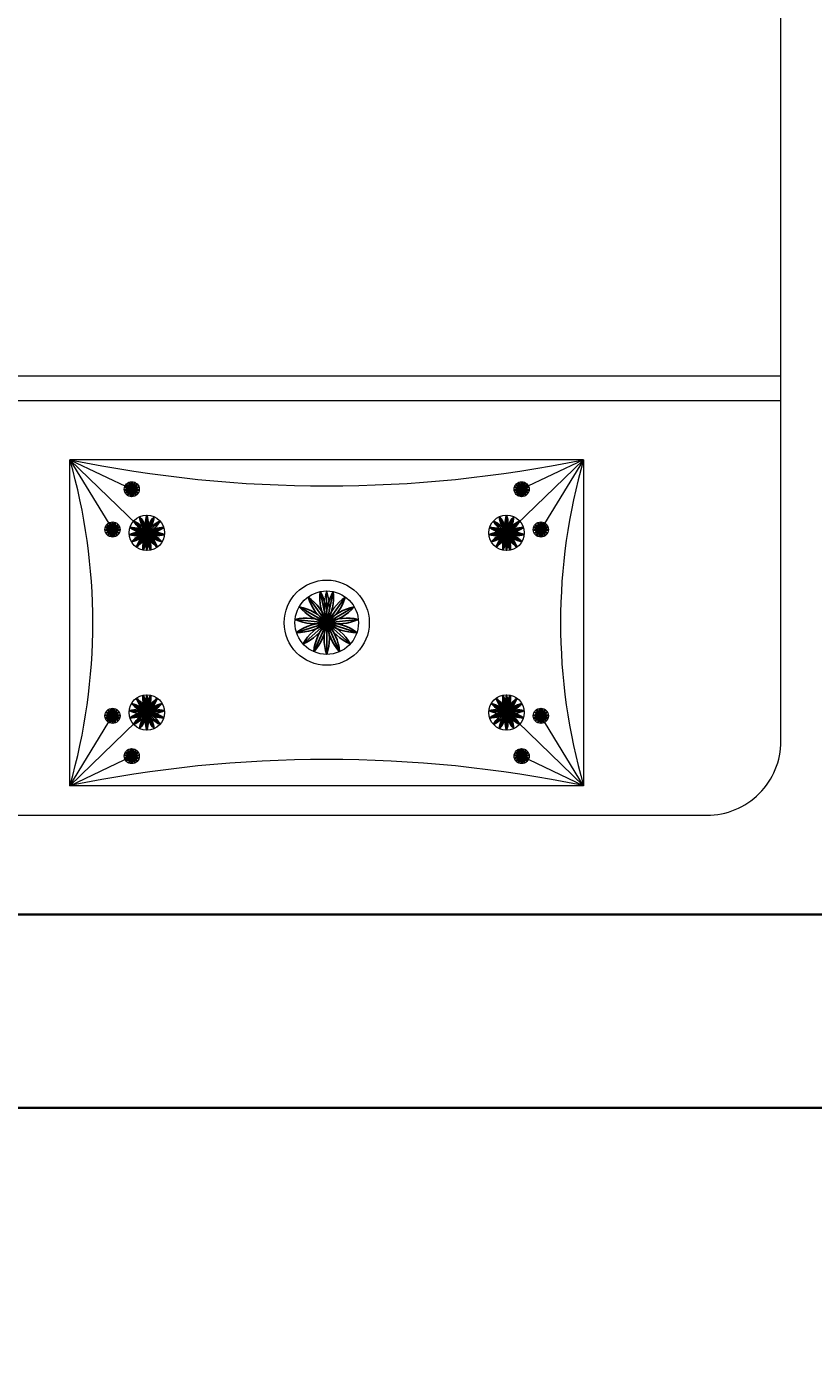
# Model space of a CAD drawing. Units: inches. Extents: x -61 to 1599, y -1316 to 257.
# Tile 187 of 204: x 1126 to 1163, y -454 to -391. Entities that reach past the tile are written whole.
import ezdxf

# ---------------------------------------------------------------- set-up
doc = ezdxf.new("R2010")
doc.units = ezdxf.units.IN
doc.header["$MEASUREMENT"] = 0
for name, color, linetype, lineweight in [('A-ANNO-DIMS', 2, 'Continuous', 18), ('FURNITURE', 83, 'Continuous', 18), ('WALLS', 4, 'Continuous', 35)]:
    doc.layers.add(name, color=color, linetype=linetype, lineweight=lineweight)
doc.layers.add('LT', color=8, linetype='Continuous')
doc.styles.get("Standard").update_dxf_attribs({"font": 'arial.ttf'})
doc.dimstyles.get("Standard").update_dxf_attribs({"dimtxt": 0.18, "dimasz": 0.18, "dimexe": 0.18, "dimexo": 0.0625, "dimgap": 0.09, "dimtad": 0, "dimtih": 1, "dimtoh": 1, "dimdec": 0, "dimzin": 0, "dimdsep": 46, "dimlunit": 3, "dimtxsty": 'Standard', "dimcen": 0.09, "dimadec": 0, "dimazin": 0, "dimtfac": 1, "dimtdec": 0, "dimtofl": 0, "dimtmove": 0, "dimatfit": 3, "dimfxl": 1, "dimtolj": 1, "dimtzin": 0, "dimarcsym": 0})

# ---------------------------------------------------------------- blocks, each defined once
blk = doc.blocks.new('*U3')
at = {"layer": 'LT'}
blk.add_line((0, 0.175), (0, -0.175), dxfattribs=at)
for centre, start, end in [((0.509, 0), 160.9983, 199.0017), ((-0.509, 0), 340.9983, 19.0017)]:
    blk.add_arc(centre, 0.539, start, end, dxfattribs=at)
blk = doc.blocks.new('*U4')
at = {"layer": 'LT', "transparency": 16777216}
for p, rotation in [((-66.649, -18.828), 96), ((-66.642, -18.755), 72), ((-66.627, -18.897), 120), ((-66.605, -18.692), 48.00000000000001), ((-66.578, -18.951), 144), ((-66.546, -18.649), 24), ((-66.512, -18.981), 168.0000000000001), ((-66.439, -18.981), 192), ((-66.404, -18.649), 336.0000000000001), ((-66.372, -18.951), 216), ((-66.345, -18.692), 312), ((-66.323, -18.897), 240), ((-66.308, -18.755), 288.0000000000001), ((-66.301, -18.828), 264)]:
    blk.add_blockref('*U3', p, dxfattribs=dict(at, rotation=rotation))
blk.add_blockref('*U3', (-66.475, -18.634), dxfattribs=at)
blk = doc.blocks.new('*U20')
at = {"layer": 'LT'}
blk.add_line((0, 0.175), (0, -0.175), dxfattribs=at)
for centre, start, end in [((0.509, 0), 160.9983, 199.0017), ((-0.509, 0), 340.9983, 19.0017)]:
    blk.add_arc(centre, 0.539, start, end, dxfattribs=at)
blk = doc.blocks.new('*U21')
at = {"layer": 'LT', "transparency": 16777216}
for p, rotation in [((-66.649, -18.828), 96), ((-66.642, -18.755), 72), ((-66.627, -18.897), 120), ((-66.605, -18.692), 48.00000000000001), ((-66.578, -18.951), 144), ((-66.546, -18.649), 24), ((-66.512, -18.981), 168.0000000000001), ((-66.439, -18.981), 192), ((-66.404, -18.649), 336.0000000000001), ((-66.372, -18.951), 216), ((-66.345, -18.692), 312), ((-66.323, -18.897), 240), ((-66.308, -18.755), 288.0000000000001), ((-66.301, -18.828), 264)]:
    blk.add_blockref('*U20', p, dxfattribs=dict(at, rotation=rotation))
blk.add_blockref('*U20', (-66.475, -18.634), dxfattribs=at)
blk = doc.blocks.new('*U52')
at = {"layer": 'LT'}
blk.add_line((0, 0.175), (0, -0.175), dxfattribs=at)
for centre, start, end in [((0.509, 0), 160.9983, 199.0017), ((-0.509, 0), 340.9983, 19.0017)]:
    blk.add_arc(centre, 0.539, start, end, dxfattribs=at)
blk = doc.blocks.new('*U53')
at = {"layer": 'LT', "transparency": 16777216}
for p, rotation in [((-66.649, -18.828), 96), ((-66.642, -18.755), 72), ((-66.627, -18.897), 120), ((-66.605, -18.692), 48.00000000000001), ((-66.578, -18.951), 144), ((-66.546, -18.649), 24), ((-66.512, -18.981), 168.0000000000001), ((-66.439, -18.981), 192), ((-66.404, -18.649), 336.0000000000001), ((-66.372, -18.951), 216), ((-66.345, -18.692), 312), ((-66.323, -18.897), 240), ((-66.308, -18.755), 288.0000000000001), ((-66.301, -18.828), 264)]:
    blk.add_blockref('*U52', p, dxfattribs=dict(at, rotation=rotation))
blk.add_blockref('*U52', (-66.475, -18.634), dxfattribs=at)
blk = doc.blocks.new('*U29')
at = {"layer": 'LT'}
blk.add_line((0, 0.175), (0, -0.175), dxfattribs=at)
for centre, start, end in [((0.509, 0), 160.9983, 199.0017), ((-0.509, 0), 340.9983, 19.0017)]:
    blk.add_arc(centre, 0.539, start, end, dxfattribs=at)
blk = doc.blocks.new('*U30')
at = {"layer": 'LT', "transparency": 16777216}
for p, rotation in [((-66.649, -18.828), 96), ((-66.642, -18.755), 72), ((-66.627, -18.897), 120), ((-66.605, -18.692), 48.00000000000001), ((-66.578, -18.951), 144), ((-66.546, -18.649), 24), ((-66.512, -18.981), 168.0000000000001), ((-66.439, -18.981), 192), ((-66.404, -18.649), 336.0000000000001), ((-66.372, -18.951), 216), ((-66.345, -18.692), 312), ((-66.323, -18.897), 240), ((-66.308, -18.755), 288.0000000000001), ((-66.301, -18.828), 264)]:
    blk.add_blockref('*U29', p, dxfattribs=dict(at, rotation=rotation))
blk.add_blockref('*U29', (-66.475, -18.634), dxfattribs=at)
blk = doc.blocks.new('*U5')
at = {"layer": 'LT'}
blk.add_line((0, 0.412), (0, -0.412), dxfattribs=at)
for centre, start, end in [((1.198, 0), 160.9983, 199.0017), ((-1.198, 0), 340.9983, 19.0017)]:
    blk.add_arc(centre, 1.267, start, end, dxfattribs=at)
blk = doc.blocks.new('*U47')
at = {"layer": 'LT', "transparency": 16777216}
for p, rotation in [((-156.639, -43.959), 48.00000000000001), ((-156.501, -43.858), 24), ((-156.165, -43.858), 336.0000000000001), ((-156.027, -43.959), 312), ((-156.743, -44.278), 96), ((-156.725, -44.108), 72), ((-156.69, -44.441), 120), ((-156.575, -44.569), 144), ((-156.419, -44.639), 168), ((-156.247, -44.639), 192), ((-156.091, -44.569), 216), ((-155.976, -44.441), 240), ((-155.941, -44.108), 288.0000000000001), ((-155.923, -44.278), 264)]:
    blk.add_blockref('*U5', p, dxfattribs=dict(at, rotation=rotation))
blk.add_blockref('*U5', (-156.333, -43.823), dxfattribs=at)
blk = doc.blocks.new('*U22')
at = {"layer": 'LT'}
blk.add_line((0, 0.412), (0, -0.412), dxfattribs=at)
for centre, start, end in [((1.198, 0), 160.9983, 199.0017), ((-1.198, 0), 340.9983, 19.0017)]:
    blk.add_arc(centre, 1.267, start, end, dxfattribs=at)
blk = doc.blocks.new('*U23')
at = {"layer": 'LT', "transparency": 16777216}
for p, rotation in [((-156.639, -43.959), 48.00000000000001), ((-156.501, -43.858), 24), ((-156.165, -43.858), 336.0000000000001), ((-156.027, -43.959), 312), ((-156.743, -44.278), 96), ((-156.725, -44.108), 72), ((-156.69, -44.441), 120), ((-156.575, -44.569), 144), ((-156.419, -44.639), 168), ((-156.247, -44.639), 192), ((-156.091, -44.569), 216), ((-155.976, -44.441), 240), ((-155.941, -44.108), 288.0000000000001), ((-155.923, -44.278), 264)]:
    blk.add_blockref('*U22', p, dxfattribs=dict(at, rotation=rotation))
blk.add_blockref('*U22', (-156.333, -43.823), dxfattribs=at)
blk = doc.blocks.new('*U54')
at = {"layer": 'LT'}
blk.add_line((0, 0.739), (0, -0.739), dxfattribs=at)
for centre, start, end in [((2.147, 0), 160.9983, 199.0017), ((-2.147, 0), 340.9983, 19.0017)]:
    blk.add_arc(centre, 2.27, start, end, dxfattribs=at)
blk = doc.blocks.new('*U41')
at = {"layer": 'LT', "transparency": 16777216}
for p, rotation in [((-280.791, -78.801), 48.00000000000001), ((-280.542, -78.621), 23.99999999999999), ((-279.941, -78.621), 336.0000000000001), ((-279.692, -78.801), 312), ((-280.945, -79.067), 72), ((-279.539, -79.067), 288.0000000000001), ((-280.977, -79.373), 96), ((-280.882, -79.665), 120), ((-280.676, -79.894), 144), ((-280.395, -80.019), 168), ((-280.088, -80.019), 191.9999999999999), ((-279.807, -79.894), 216), ((-279.602, -79.665), 240), ((-279.507, -79.373), 264)]:
    blk.add_blockref('*U54', p, dxfattribs=dict(at, rotation=rotation))
blk.add_blockref('*U54', (-280.242, -78.557), dxfattribs=at)
blk = doc.blocks.new('*U42')
at = {"layer": 'LT'}
blk.add_line((0, 0.412), (0, -0.412), dxfattribs=at)
for centre, start, end in [((1.198, 0), 160.9983, 199.0017), ((-1.198, 0), 340.9983, 19.0017)]:
    blk.add_arc(centre, 1.267, start, end, dxfattribs=at)
blk = doc.blocks.new('*U43')
at = {"layer": 'LT', "transparency": 16777216}
for p, rotation in [((-156.639, -43.959), 48.00000000000001), ((-156.501, -43.858), 24), ((-156.165, -43.858), 336.0000000000001), ((-156.027, -43.959), 312), ((-156.743, -44.278), 96), ((-156.725, -44.108), 72), ((-156.69, -44.441), 120), ((-156.575, -44.569), 144), ((-156.419, -44.639), 168), ((-156.247, -44.639), 192), ((-156.091, -44.569), 216), ((-155.976, -44.441), 240), ((-155.941, -44.108), 288.0000000000001), ((-155.923, -44.278), 264)]:
    blk.add_blockref('*U42', p, dxfattribs=dict(at, rotation=rotation))
blk.add_blockref('*U42', (-156.333, -43.823), dxfattribs=at)
blk = doc.blocks.new('*U31')
at = {"layer": 'LT'}
blk.add_line((0, 0.412), (0, -0.412), dxfattribs=at)
for centre, start, end in [((1.198, 0), 160.9983, 199.0017), ((-1.198, 0), 340.9983, 19.0017)]:
    blk.add_arc(centre, 1.267, start, end, dxfattribs=at)
blk = doc.blocks.new('*U32')
at = {"layer": 'LT', "transparency": 16777216}
for p, rotation in [((-156.639, -43.959), 48.00000000000001), ((-156.501, -43.858), 24), ((-156.165, -43.858), 336.0000000000001), ((-156.027, -43.959), 312), ((-156.743, -44.278), 96), ((-156.725, -44.108), 72), ((-156.69, -44.441), 120), ((-156.575, -44.569), 144), ((-156.419, -44.639), 168), ((-156.247, -44.639), 192), ((-156.091, -44.569), 216), ((-155.976, -44.441), 240), ((-155.941, -44.108), 288.0000000000001), ((-155.923, -44.278), 264)]:
    blk.add_blockref('*U31', p, dxfattribs=dict(at, rotation=rotation))
blk.add_blockref('*U31', (-156.333, -43.823), dxfattribs=at)
blk = doc.blocks.new('*U48')
at = {"layer": 'LT'}
blk.add_line((0, 0.175), (0, -0.175), dxfattribs=at)
for centre, start, end in [((0.509, 0), 160.9983, 199.0017), ((-0.509, 0), 340.9983, 19.0017)]:
    blk.add_arc(centre, 0.539, start, end, dxfattribs=at)
blk = doc.blocks.new('*U49')
at = {"layer": 'LT', "transparency": 16777216}
for p, rotation in [((-66.649, -18.828), 96), ((-66.642, -18.755), 72), ((-66.627, -18.897), 120), ((-66.605, -18.692), 48.00000000000001), ((-66.578, -18.951), 144), ((-66.546, -18.649), 24), ((-66.512, -18.981), 168.0000000000001), ((-66.439, -18.981), 192), ((-66.404, -18.649), 336.0000000000001), ((-66.372, -18.951), 216), ((-66.345, -18.692), 312), ((-66.323, -18.897), 240), ((-66.308, -18.755), 288.0000000000001), ((-66.301, -18.828), 264)]:
    blk.add_blockref('*U48', p, dxfattribs=dict(at, rotation=rotation))
blk.add_blockref('*U48', (-66.475, -18.634), dxfattribs=at)
blk = doc.blocks.new('*U24')
at = {"layer": 'LT'}
blk.add_line((0, 0.175), (0, -0.175), dxfattribs=at)
for centre, start, end in [((0.509, 0), 160.9983, 199.0017), ((-0.509, 0), 340.9983, 19.0017)]:
    blk.add_arc(centre, 0.539, start, end, dxfattribs=at)
blk = doc.blocks.new('*U25')
at = {"layer": 'LT', "transparency": 16777216}
for p, rotation in [((-66.649, -18.828), 96), ((-66.642, -18.755), 72), ((-66.627, -18.897), 120), ((-66.605, -18.692), 48.00000000000001), ((-66.578, -18.951), 144), ((-66.546, -18.649), 24), ((-66.512, -18.981), 168.0000000000001), ((-66.439, -18.981), 192), ((-66.404, -18.649), 336.0000000000001), ((-66.372, -18.951), 216), ((-66.345, -18.692), 312), ((-66.323, -18.897), 240), ((-66.308, -18.755), 288.0000000000001), ((-66.301, -18.828), 264)]:
    blk.add_blockref('*U24', p, dxfattribs=dict(at, rotation=rotation))
blk.add_blockref('*U24', (-66.475, -18.634), dxfattribs=at)
blk = doc.blocks.new('*U50')
at = {"layer": 'LT'}
blk.add_line((0, 0.175), (0, -0.175), dxfattribs=at)
for centre, start, end in [((0.509, 0), 160.9983, 199.0017), ((-0.509, 0), 340.9983, 19.0017)]:
    blk.add_arc(centre, 0.539, start, end, dxfattribs=at)
blk = doc.blocks.new('*U51')
at = {"layer": 'LT', "transparency": 16777216}
for p, rotation in [((-66.649, -18.828), 96), ((-66.642, -18.755), 72), ((-66.627, -18.897), 120), ((-66.605, -18.692), 48.00000000000001), ((-66.578, -18.951), 144), ((-66.546, -18.649), 24), ((-66.512, -18.981), 168.0000000000001), ((-66.439, -18.981), 192), ((-66.404, -18.649), 336.0000000000001), ((-66.372, -18.951), 216), ((-66.345, -18.692), 312), ((-66.323, -18.897), 240), ((-66.308, -18.755), 288.0000000000001), ((-66.301, -18.828), 264)]:
    blk.add_blockref('*U50', p, dxfattribs=dict(at, rotation=rotation))
blk.add_blockref('*U50', (-66.475, -18.634), dxfattribs=at)
blk = doc.blocks.new('*U26')
at = {"layer": 'LT'}
blk.add_line((0, 0.175), (0, -0.175), dxfattribs=at)
for centre, start, end in [((0.509, 0), 160.9983, 199.0017), ((-0.509, 0), 340.9983, 19.0017)]:
    blk.add_arc(centre, 0.539, start, end, dxfattribs=at)
blk = doc.blocks.new('*U27')
at = {"layer": 'LT', "transparency": 16777216}
for p, rotation in [((-66.649, -18.828), 96), ((-66.642, -18.755), 72), ((-66.627, -18.897), 120), ((-66.605, -18.692), 48.00000000000001), ((-66.578, -18.951), 144), ((-66.546, -18.649), 24), ((-66.512, -18.981), 168.0000000000001), ((-66.439, -18.981), 192), ((-66.404, -18.649), 336.0000000000001), ((-66.372, -18.951), 216), ((-66.345, -18.692), 312), ((-66.323, -18.897), 240), ((-66.308, -18.755), 288.0000000000001), ((-66.301, -18.828), 264)]:
    blk.add_blockref('*U26', p, dxfattribs=dict(at, rotation=rotation))
blk.add_blockref('*U26', (-66.475, -18.634), dxfattribs=at)
blk = doc.blocks.new('BED-DOUBLE')
for p, q in [((1.272, 20.467), (70.263, 20.467)), ((1.272, 19.317), (70.263, 19.317)), ((37.147, 1.379), (37.147, 16.557)), ((61.064, 16.557), (37.147, 16.557)), ((37.147, 16.557), (40.027, 15.18)), ((37.147, 16.557), (40.715, 13.107)), ((37.147, 16.557), (39.13, 13.305)), ((61.064, 16.557), (57.496, 13.107)), ((61.064, 16.557), (58.185, 15.18)), ((61.064, 16.557), (59.081, 13.305)), ((40.027, 15.18), (40.027, 14.829)), ((58.185, 15.18), (58.185, 14.829)), ((39.13, 13.305), (39.13, 12.955)), ((59.081, 13.305), (59.081, 12.955)), ((40.729, 13.149), (40.729, 12.324)), ((57.483, 13.149), (57.483, 12.324)), ((49.106, 8.968), (49.106, 10.447)), ((40.729, 4.788), (40.729, 5.613)), ((57.483, 4.788), (57.483, 5.613)), ((37.147, 1.379), (40.715, 4.83)), ((37.147, 1.379), (39.13, 4.631)), ((39.13, 4.631), (39.13, 4.982)), ((61.064, 1.379), (57.496, 4.83)), ((59.081, 4.631), (59.081, 4.982)), ((61.064, 1.379), (59.081, 4.631)), ((37.147, 1.379), (40.027, 2.756)), ((40.027, 2.756), (40.027, 3.107)), ((58.185, 2.756), (58.185, 3.107)), ((61.064, 1.379), (58.185, 2.756)), ((61.064, 1.379), (61.064, 1.379))]:
    blk.add_line(p, q)
for points in [[(1.272, 88.537), (1.272, 3.449, 0.414214), (4.722, 0), (66.813, 0, 0.414214), (70.263, 3.449), (70.263, 88.537, 0.414214), (66.813, 91.987), (4.722, 91.987, 0.414214)], [(40.027, 15.18, 0.167358), (40.027, 14.829, 0.167358)], [(39.13, 13.305, 0.167358), (39.13, 12.955, 0.167358)], [(59.081, 12.955, 0.167358), (59.081, 13.305, 0.167358)], [(40.729, 13.149, 0.167358), (40.729, 12.324, 0.167358)], [(57.483, 12.324, 0.167358), (57.483, 13.149, 0.167358)], [(49.106, 8.968, 0.167358), (49.106, 10.447, 0.167358)], [(40.729, 5.613, 0.167358), (40.729, 4.788, 0.167358)], [(57.483, 4.788, 0.167358), (57.483, 5.613, 0.167358)], [(39.13, 4.982, 0.167358), (39.13, 4.631, 0.167358)], [(59.081, 4.631, 0.167358), (59.081, 4.982, 0.167358)], [(40.027, 3.107, 0.167358), (40.027, 2.756, 0.167358)], [(58.185, 2.756, 0.167358), (58.185, 3.107, 0.167358)]]:
    blk.add_lwpolyline(points, format="xyb", close=True)
blk.add_lwpolyline([(61.064, 16.557), (61.064, 1.379), (37.147, 1.379)])
for centre, radius in [((40.027, 15.18), 0.351), ((58.185, 15.18), 0.351), ((40.729, 13.149), 0.825), ((57.483, 13.149), 0.825), ((39.13, 13.305), 0.351), ((59.081, 13.305), 0.351), ((49.106, 8.968), 1.982), ((49.106, 8.968), 1.478), ((40.729, 4.788), 0.825), ((57.483, 4.788), 0.825), ((39.13, 4.631), 0.351), ((59.081, 4.631), 0.351), ((40.027, 2.756), 0.351), ((58.185, 2.756), 0.351)]:
    blk.add_circle(centre, radius)
for centre, radius, start, end in [((10.674, 8.968), 27.54, 344.0046, 15.9954), ((49.106, 74.54), 59.203, 258.34678, 281.65322), ((87.538, 8.968), 27.54, 164.0046, 195.9954), ((58.694, 15.005), 0.539, 160.9983, 199.0017), ((57.675, 15.005), 0.539, 340.9983, 19.0017), ((49.106, -56.603), 59.203, 78.34678, 101.65322)]:
    blk.add_arc(centre, radius, start, end)
for name, p in [('*U30', (106.502, 33.99)), ('*U23', (197.062, 57.384)), ('*U21', (105.605, 32.115))]:
    blk.add_blockref(name, p)
at = {"extrusion": (0, 0, -1), "zscale": -1}
for name, p in [('*U25', (8.291, 33.99)), ('*U32', (98.85, 57.384)), ('*U27', (7.394, 32.115))]:
    blk.add_blockref(name, p, dxfattribs=at)
at = {"rotation": 180}
for name, p in [('*U41', (-231.136, -70.328)), ('*U43', (-98.85, -39.447)), ('*U51', (-7.394, -14.178)), ('*U49', (-8.291, -16.053))]:
    blk.add_blockref(name, p, dxfattribs=at)
at = {"extrusion": (0, 0, -1), "zscale": -1, "rotation": 180}
for name, p in [('*U47', (-197.062, -39.447)), ('*U4', (-105.605, -14.178)), ('*U53', (-106.502, -16.053))]:
    blk.add_blockref(name, p, dxfattribs=at)
blk = doc.blocks.new('*D698')
at = {"layer": 'A-ANNO-DIMS', "color": 0, "lineweight": -2, "transparency": 16777216}
for p, q in [((644.765, -167.169), (1598.483, -167.169)), ((1598.303, -167.349), (1598.303, -363.987)), ((1598.303, -560.989), (1598.303, -364.351)), ((644.765, -561.169), (1598.483, -561.169))]:
    blk.add_line(p, q, dxfattribs=at)
at = {"layer": 'A-ANNO-DIMS', "color": 0, "transparency": 16777216}
for points in [[(1598.273, -167.349), (1598.333, -167.349), (1598.303, -167.169)], [(1598.273, -560.989), (1598.333, -560.989), (1598.303, -561.169)]]:
    blk.add_solid(points, dxfattribs=at)
at = {"layer": 'DEFPOINTS', "color": 0, "transparency": 16777216}
for p in [(644.703, -167.169), (1598.303, -167.169), (644.703, -561.169)]:
    blk.add_point(p, dxfattribs=at)
at = {"layer": 'A-ANNO-DIMS', "color": 0, "transparency": 16777216, "insert": (1598.303, -364.169), "char_height": 0.18, "attachment_point": 5}
blk.add_mtext('\\A1;394', dxfattribs=at)

msp = doc.modelspace()

# ---------------------------------------------------------------- linework, layer by layer
at = {"layer": 'WALLS'}
for p, q in [((1065.7028, -432.3229), (1215.7028, -432.3229)), ((992.7028, -441.3229), (1215.7028, -441.3229))]:
    msp.add_line(p, q, dxfattribs=at)

# ---------------------------------------------------------------- block references
at = {"layer": 'FURNITURE'}
msp.add_blockref('BED-DOUBLE', (1091.2612, -427.6961), dxfattribs=at)

# ---------------------------------------------------------------- dimensions: what is measured, and where the dimension line sits
at = {"layer": 'A-ANNO-DIMS'}
dim = msp.add_linear_dim(base=(1598.3028, -167.169), p1=(644.7028, -561.169), p2=(644.7028, -167.169), angle=90, dimstyle='Standard', override={"dimdec": 0, "dimlfac": 1, "dimrnd": 0, "dimzin": 0, "dimdsep": 46, "dimlunit": 2}, dxfattribs=at)
dim.commit()
dim.dimension.update_dxf_attribs({"geometry": '*D698', "text_midpoint": (1598.3028, -364.169)})

doc.saveas('drawing.dxf')
